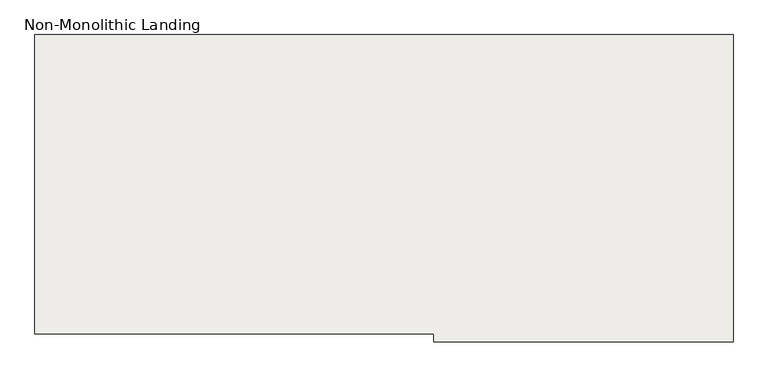
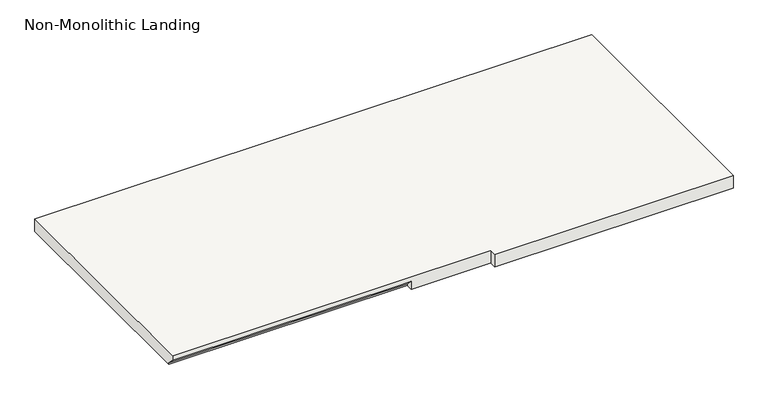
"""IFC4 building model written with IfcOpenShell, lengths in millimetres: slab geometry, Non-Monolithic Landing."""

from ifc_helpers import new_model, si_unit, origin, place, context, project, spatial, faceted_brep, source, transform, mapped, element, save


def non_monolithic_landing_d45999a6(model_context):
    return source(origin(), model_context, "Body", "Brep", [
        faceted_brep([(-3617.4415084, 23194.7216096, 36560.9005799), (-3617.4415084, 23220.1216096, 36535.5005799), (-2703.0415084, 23220.1216096, 36535.5005799), (-2703.0415084, 23194.7216096, 36560.9005799), (-2398.2415084, 23194.7216096, 36579.9505799), (-2398.2415084, 23169.3216096, 36579.9505799), (-1483.8415084, 23169.3216096, 36579.9505799), (-1483.8415084, 23194.7216096, 36579.9505799), (-1483.8415084, 24109.1216096, 36579.9505799), (-3617.4415084, 24109.1216096, 36579.9505799), (-3617.4415084, 23194.7216096, 36579.9505799), (-2703.0415084, 23220.1216096, 36529.1505799), (-3617.4415084, 23220.1216096, 36529.1505799), (-3617.4415084, 24109.1216096, 36529.1505799), (-1483.8415084, 24109.1216096, 36529.1505799), (-1483.8415084, 23194.7216096, 36529.1505799), (-1483.8415084, 23169.3216096, 36529.1505799), (-2398.2415084, 23169.3216096, 36529.1505799), (-2398.2415084, 23194.7216096, 36529.1505799), (-2703.0415084, 23194.7216096, 36529.1505799)], [[[0, 1, 2, 3]], [[4, 5, 6, 7, 8, 9, 10]], [[11, 12, 13, 14, 15, 16, 17, 18, 19]], [[12, 11, 2, 1]], [[11, 19, 3, 2]], [[4, 10, 0, 3, 19, 18]], [[5, 4, 18, 17]], [[6, 5, 17, 16]], [[7, 6, 16, 15]], [[8, 7, 15, 14]], [[9, 8, 14, 13]], [[10, 9, 13, 12, 1, 0]]]),
    ])


if __name__ == "__main__":
    model = new_model("IFC4")
    model_context = context("Model", 3, world=origin())
    ifc_project = project(units=[si_unit("LENGTHUNIT", "METRE", prefix="MILLI")], contexts=[model_context])
    site = spatial("IfcSite", under=ifc_project)
    building = spatial("IfcBuilding", under=site)
    placement = place(None, origin())
    non_monolithic_landing_shape = non_monolithic_landing_d45999a6(model_context)
    element("IfcSlab", 1, ObjectType="Non-Monolithic Landing", at=placement, inside=building, context=model_context, shape_type="MappedRepresentation", body=[
        mapped(non_monolithic_landing_shape, transform((0.0, 0.0, 0.0), x_axis=(1.0, 0.0, 0.0), y_axis=(0.0, 1.0, 0.0), z_axis=(0.0, 0.0, 1.0))),
    ])
    save(model, "model.ifc")
